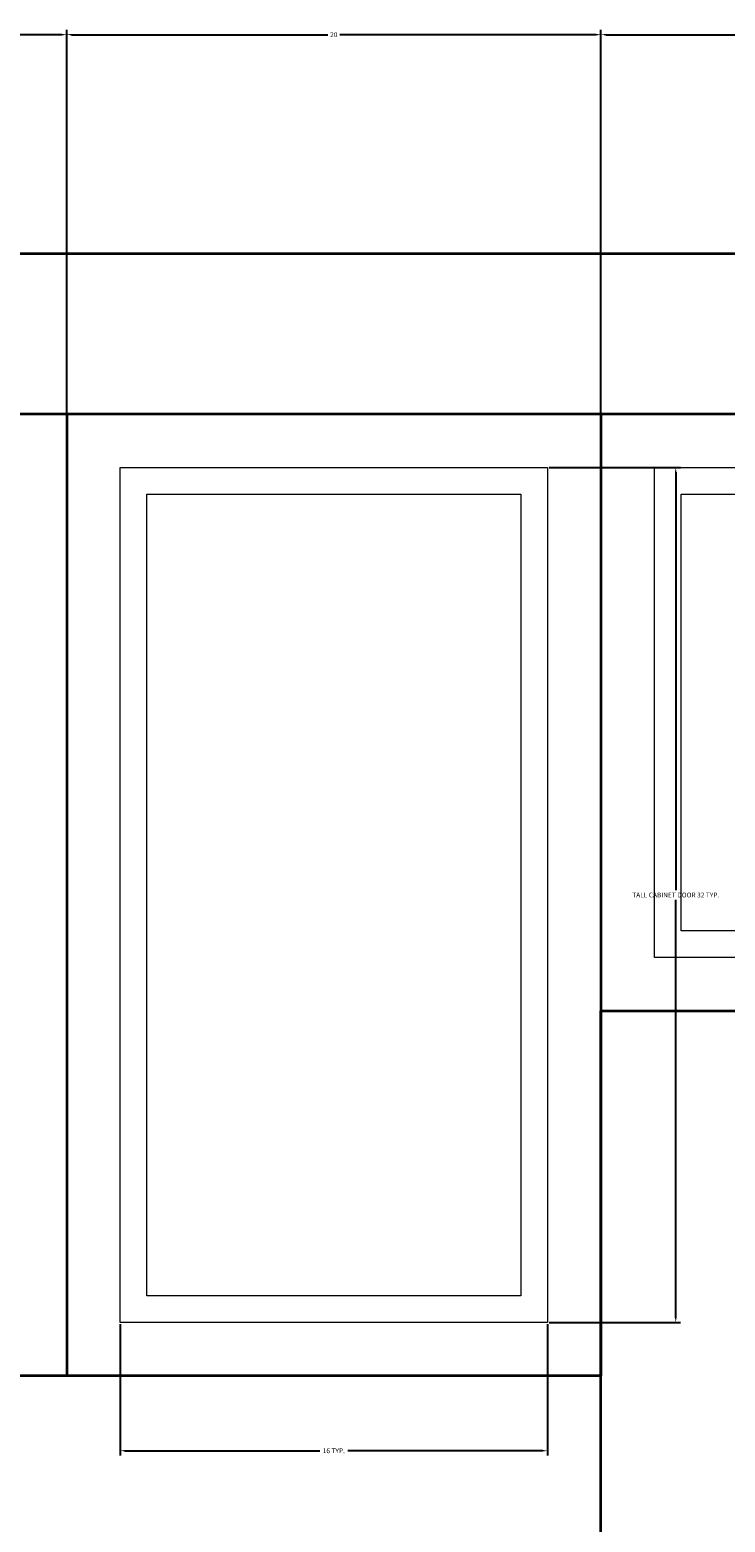
# Model space of a CAD drawing. Units: inches. Extents: x 27 to 200, y -50 to 102.
# Tile 7 of 26: x 63 to 89, y 46 to 102. Entities that reach past the tile are written whole.
import ezdxf

# ---------------------------------------------------------------- set-up
doc = ezdxf.new("R2010")
doc.units = ezdxf.units.IN
doc.header["$MEASUREMENT"] = 0
for name, color, linetype, lineweight in [('A-ANNO-DIMS', 2, 'Continuous', 18), ('A-ELEV', 7, 'Continuous', 35), ('A-FURN', 8, 'Continuous', 18)]:
    doc.layers.add(name, color=color, linetype=linetype, lineweight=lineweight)
doc.styles.get("Standard").update_dxf_attribs({"font": 'arial.ttf'})
doc.dimstyles.get("Standard").update_dxf_attribs({"dimtxt": 0.18, "dimasz": 0.18, "dimexe": 0.18, "dimexo": 0.0625, "dimgap": 0.09, "dimtad": 0, "dimtih": 1, "dimtoh": 1, "dimdec": 4, "dimzin": 0, "dimdsep": 46, "dimtxsty": 'Standard', "dimcen": 0.09, "dimadec": 0, "dimazin": 0, "dimtfac": 1, "dimtdec": 4, "dimtofl": 0, "dimtmove": 0, "dimatfit": 3, "dimfxl": 1, "dimtolj": 1, "dimtzin": 0, "dimarcsym": 0})

# ---------------------------------------------------------------- blocks, each defined once
blk = doc.blocks.new('CAB-DOOR-UPPER')
for p, q in [((0, 0), (0, 18.339)), ((0, 18.339), (14, 18.339)), ((14, 18.339), (14, 0)), ((1, 1), (1, 17.339)), ((1, 17.339), (13, 17.339)), ((13, 17.339), (13, 1)), ((13, 1), (1, 1)), ((14, 0), (0, 0))]:
    blk.add_line(p, q)
blk = doc.blocks.new('CAB-DOOR-TALL')
for p, q in [((0, 0), (0, 32)), ((0, 32), (16, 32)), ((16, 32), (16, 0)), ((1, 1), (1, 31)), ((1, 31), (15, 31)), ((15, 31), (15, 1)), ((15, 1), (1, 1)), ((16, 0), (0, 0))]:
    blk.add_line(p, q)
blk = doc.blocks.new('*D7')
at = {"layer": 'A-ANNO-DIMS', "color": 0, "lineweight": -2, "transparency": 16777216}
for p, q in [((82.479, 85.926), (87.397, 85.926)), ((87.217, 85.746), (87.217, 70.11)), ((87.217, 54.106), (87.217, 69.743)), ((82.479, 53.926), (87.397, 53.926))]:
    blk.add_line(p, q, dxfattribs=at)
at = {"layer": 'A-ANNO-DIMS', "color": 0, "transparency": 16777216}
for points in [[(87.187, 85.746), (87.247, 85.746), (87.217, 85.926)], [(87.187, 54.106), (87.247, 54.106), (87.217, 53.926)]]:
    blk.add_solid(points, dxfattribs=at)
at = {"layer": 'Defpoints', "color": 0, "transparency": 16777216}
for p in [(82.417, 85.926), (87.217, 85.926), (82.417, 53.926)]:
    blk.add_point(p, dxfattribs=at)
at = {"layer": 'A-ANNO-DIMS', "color": 0, "transparency": 16777216, "insert": (87.217, 69.926), "char_height": 0.18, "attachment_point": 5}
blk.add_mtext('\\A1;TALL CABINET DOOR 32 TYP.', dxfattribs=at)
blk = doc.blocks.new('*D8')
at = {"layer": 'A-ANNO-DIMS', "color": 0, "lineweight": -2, "transparency": 16777216}
for p, q in [((66.417, 53.864), (66.417, 48.946)), ((82.417, 53.864), (82.417, 48.946)), ((66.597, 49.126), (73.897, 49.126)), ((82.237, 49.126), (74.937, 49.126))]:
    blk.add_line(p, q, dxfattribs=at)
at = {"layer": 'A-ANNO-DIMS', "color": 0, "transparency": 16777216}
for points in [[(66.597, 49.156), (66.597, 49.096), (66.417, 49.126)], [(82.237, 49.156), (82.237, 49.096), (82.417, 49.126)]]:
    blk.add_solid(points, dxfattribs=at)
at = {"layer": 'Defpoints', "color": 0, "transparency": 16777216}
for p in [(66.417, 53.926), (82.417, 53.926), (82.417, 49.126)]:
    blk.add_point(p, dxfattribs=at)
at = {"layer": 'A-ANNO-DIMS', "color": 0, "transparency": 16777216, "insert": (74.417, 49.126), "char_height": 0.18, "attachment_point": 5}
blk.add_mtext('\\A1;16 TYP.', dxfattribs=at)
blk = doc.blocks.new('*D14')
at = {"layer": 'A-ANNO-DIMS', "color": 0, "lineweight": -2, "transparency": 16777216}
for p, q in [((44.417, 87.989), (44.417, 102.306)), ((64.417, 87.989), (64.417, 102.306)), ((44.597, 102.126), (54.197, 102.126)), ((64.237, 102.126), (54.637, 102.126))]:
    blk.add_line(p, q, dxfattribs=at)
at = {"layer": 'A-ANNO-DIMS', "color": 0, "transparency": 16777216}
for points in [[(44.597, 102.156), (44.597, 102.096), (44.417, 102.126)], [(64.237, 102.156), (64.237, 102.096), (64.417, 102.126)]]:
    blk.add_solid(points, dxfattribs=at)
at = {"layer": 'Defpoints', "color": 0, "transparency": 16777216}
for p in [(64.417, 102.126), (44.417, 87.926), (64.417, 87.926)]:
    blk.add_point(p, dxfattribs=at)
at = {"layer": 'A-ANNO-DIMS', "color": 0, "transparency": 16777216, "insert": (54.417, 102.126), "char_height": 0.18, "attachment_point": 5}
blk.add_mtext('\\A1;20', dxfattribs=at)
blk = doc.blocks.new('*D15')
at = {"layer": 'A-ANNO-DIMS', "color": 0, "lineweight": -2, "transparency": 16777216}
for p, q in [((64.417, 87.989), (64.417, 102.306)), ((84.417, 87.989), (84.417, 102.306)), ((64.597, 102.126), (74.197, 102.126)), ((84.237, 102.126), (74.637, 102.126))]:
    blk.add_line(p, q, dxfattribs=at)
at = {"layer": 'A-ANNO-DIMS', "color": 0, "transparency": 16777216}
for points in [[(64.597, 102.156), (64.597, 102.096), (64.417, 102.126)], [(84.237, 102.156), (84.237, 102.096), (84.417, 102.126)]]:
    blk.add_solid(points, dxfattribs=at)
at = {"layer": 'Defpoints', "color": 0, "transparency": 16777216}
for p in [(84.417, 102.126), (64.417, 87.926), (84.417, 87.926)]:
    blk.add_point(p, dxfattribs=at)
at = {"layer": 'A-ANNO-DIMS', "color": 0, "transparency": 16777216, "insert": (74.417, 102.126), "char_height": 0.18, "attachment_point": 5}
blk.add_mtext('\\A1;20', dxfattribs=at)
blk = doc.blocks.new('*D16')
at = {"layer": 'A-ANNO-DIMS', "color": 0, "lineweight": -2, "transparency": 16777216}
for p, q in [((84.417, 87.989), (84.417, 102.306)), ((102.417, 87.989), (102.417, 102.306)), ((84.597, 102.126), (93.206, 102.126)), ((102.237, 102.126), (93.628, 102.126))]:
    blk.add_line(p, q, dxfattribs=at)
at = {"layer": 'A-ANNO-DIMS', "color": 0, "transparency": 16777216}
for points in [[(84.597, 102.156), (84.597, 102.096), (84.417, 102.126)], [(102.237, 102.156), (102.237, 102.096), (102.417, 102.126)]]:
    blk.add_solid(points, dxfattribs=at)
at = {"layer": 'Defpoints', "color": 0, "transparency": 16777216}
for p in [(102.417, 102.126), (84.417, 87.926), (102.417, 87.926)]:
    blk.add_point(p, dxfattribs=at)
at = {"layer": 'A-ANNO-DIMS', "color": 0, "transparency": 16777216, "insert": (93.417, 102.126), "char_height": 0.18, "attachment_point": 5}
blk.add_mtext('\\A1;18', dxfattribs=at)

msp = doc.modelspace()

# ---------------------------------------------------------------- linework, layer by layer
at = {"layer": 'A-ELEV'}
for p, q in [((191.4169, 93.9264), (35.4169, 93.9264)), ((191.4169, 87.9264), (35.4169, 87.9264)), ((64.4169, 87.9264), (64.4169, 51.9264)), ((84.4169, 87.9264), (84.4169, 51.9264)), ((84.4169, 65.5865), (120.4169, 65.5865)), ((84.4169, 51.9264), (44.4169, 51.9264))]:
    msp.add_line(p, q, dxfattribs=at)
msp.add_lwpolyline([(84.4169, 65.5865), (120.4169, 65.5865), (120.4169, 39.8559), (84.4169, 39.8559)], close=True, dxfattribs=at)

# ---------------------------------------------------------------- block references
at = {"layer": 'A-FURN'}
for name, p in [('CAB-DOOR-TALL', (66.417, 53.926)), ('CAB-DOOR-UPPER', (86.417, 67.587))]:
    msp.add_blockref(name, p, dxfattribs=at)

# ---------------------------------------------------------------- dimensions: what is measured, and where the dimension line sits
at = {"layer": 'A-ANNO-DIMS'}
for base, p1, p2, picture, middle in [((64.4169, 102.1264), (44.4169, 87.9264), (64.4169, 87.9264), '*D14', (54.4169, 102.1264)), ((84.4169, 102.1264), (64.4169, 87.9264), (84.4169, 87.9264), '*D15', (74.4169, 102.1264)), ((102.4169, 102.1264), (84.4169, 87.9264), (102.4169, 87.9264), '*D16', (93.4169, 102.1264))]:
    dim = msp.add_linear_dim(base=base, p1=p1, p2=p2, dimstyle='Standard', override={"dimdec": 0, "dimlfac": 1, "dimrnd": 0, "dimzin": 0, "dimdsep": 46, "dimlunit": 2}, dxfattribs=at)
    dim.commit()
    dim.dimension.update_dxf_attribs({"geometry": picture, "text_midpoint": middle})
dim = msp.add_linear_dim(base=(87.2169, 85.9264), p1=(82.4169, 53.9264), p2=(82.4169, 85.9264), angle=90, text='TALL CABINET DOOR <> TYP.', dimstyle='Standard', override={"dimdec": 0, "dimrnd": 0, "dimzin": 0, "dimlunit": 2}, dxfattribs=at)
dim.commit()
dim.dimension.update_dxf_attribs({"geometry": '*D7', "text_midpoint": (87.2169, 69.9264)})
dim = msp.add_linear_dim(base=(82.4169, 49.1264), p1=(66.4169, 53.9264), p2=(82.4169, 53.9264), text='<> TYP.', dimstyle='Standard', override={"dimdec": 0, "dimrnd": 0, "dimzin": 0, "dimlunit": 2}, dxfattribs=at)
dim.commit()
dim.dimension.update_dxf_attribs({"geometry": '*D8', "text_midpoint": (74.4169, 49.1264)})

doc.saveas('drawing.dxf')
